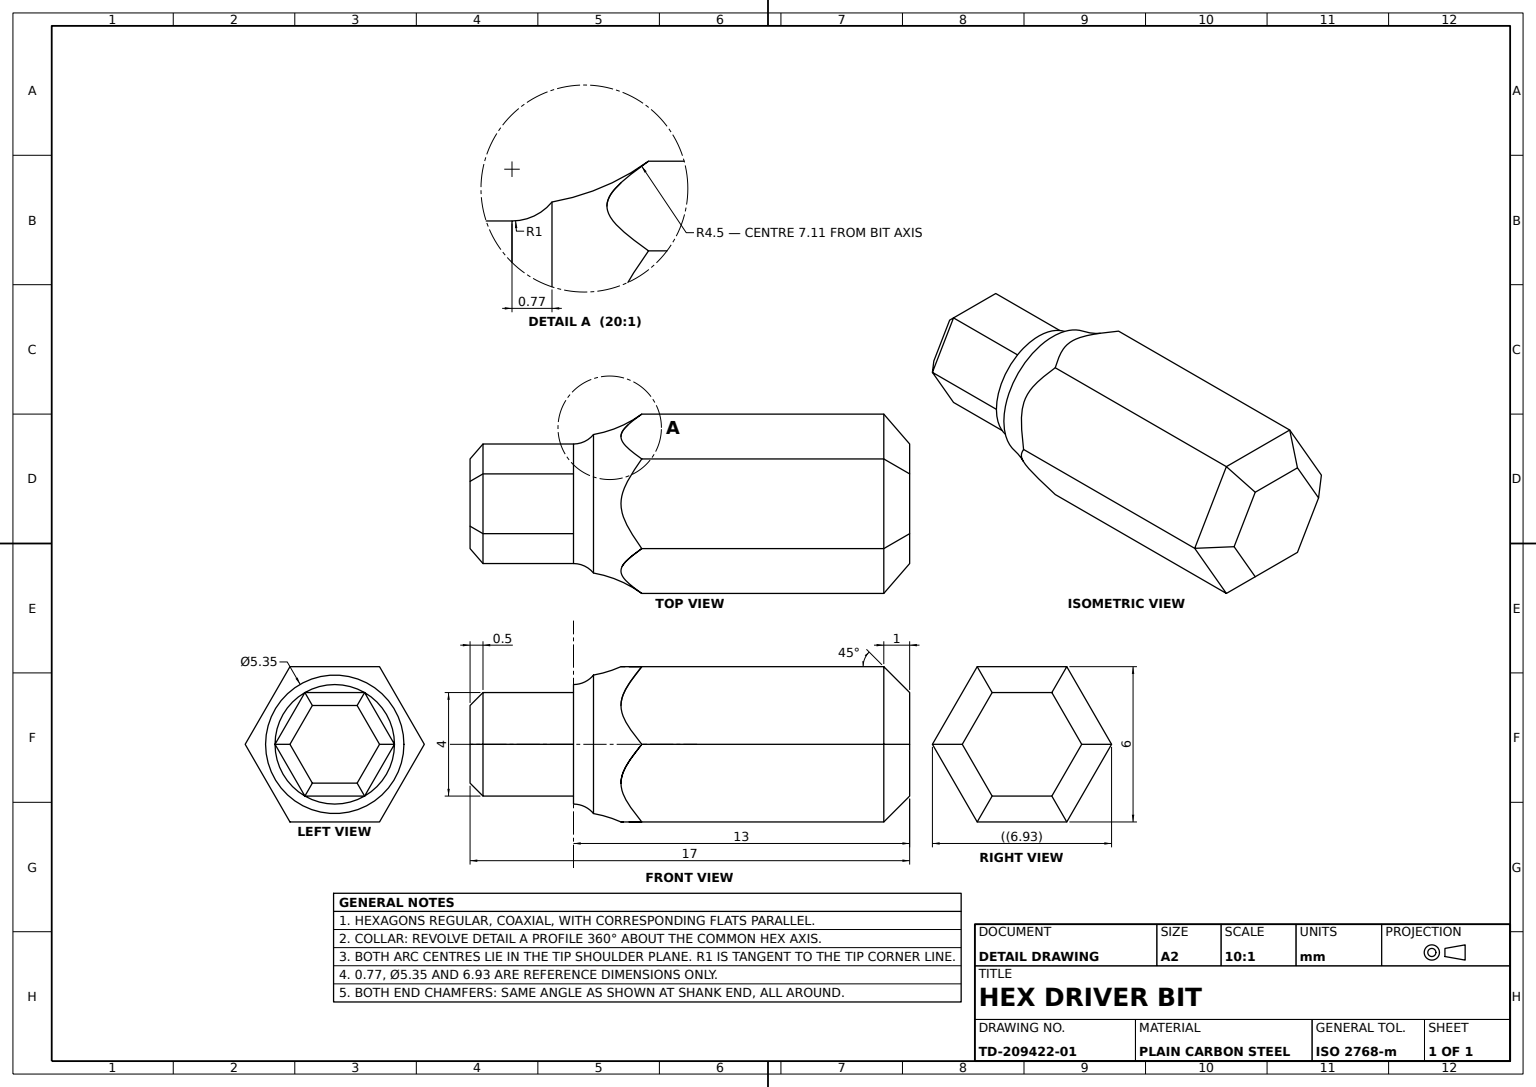
SolidWorks part; units mm, degrees
material "Plain Carbon Steel"
ref_plane "Front Plane" through (0, 0, 0) normal (0, 0, 1) x (1, 0, 0)
ref_plane "Top Plane" through (0, 0, 0) normal (0, 1, 0) x (1, 0, 0)
ref_plane "Right Plane" through (0, 0, 0) normal (1, 0, 0) x (0, 0, -1)
sketch "Hex Shank Profile 6AF" plane through (0, 0, 0) normal (0, 0, 1) x (1, 0, 0)
  line L1 (3.4641, 0) -> (1.7321, 3)
  line L2 (1.7321, 3) -> (-1.7321, 3)
  line L3 (-1.7321, 3) -> (-3.4641, 0)
  line L4 (-3.4641, 0) -> (-1.7321, -3)
  line L5 (-1.7321, -3) -> (1.7321, -3)
  line L6 (1.7321, -3) -> (3.4641, 0)
  circle A0 centre (0, 0) radius 3 construction
  dimension "D1" = 6
extrude "Hex Shank 6AF x13" add sketch "Hex Shank Profile 6AF" along normal blind 13
sketch "Hex Tip Profile 4AF" plane through (0, 0, 13) normal (0, 0, 1) x (1, 0, 0)
  line L1 (2.3094, 0) -> (1.1547, 2)
  line L2 (1.1547, 2) -> (-1.1547, 2)
  line L3 (-1.1547, 2) -> (-2.3094, 0)
  line L4 (-2.3094, 0) -> (-1.1547, -2)
  line L5 (-1.1547, -2) -> (1.1547, -2)
  line L6 (1.1547, -2) -> (2.3094, 0)
  circle A0 centre (0, 0) radius 2 construction
  dimension "D1" = 4
extrude "Hex Tip 4AF x4" add sketch "Hex Tip Profile 4AF" along normal blind 4 and the other way blind 4
sketch "Neck Groove Profile" plane through (0, 0, 0) normal (0, 1, 0) x (1, 0, 0)
  line L4 (3.4641, -10.3601) -> (3.4641, -13)
  line L15 (3.4641, -13) -> (3.4641, 0) construction
  line L32 (0, 0) -> (0, -2.2545) construction
  line L34 (1.1547, -17) -> (2.3094, -17) construction
  line L35 (2.3094, -13) -> (3.4641, -13)
  line L40 (2.3094, -13) -> (2.3094, -17) construction
  arc A1 (2.6753, -12.2267) -> (3.4641, -10.3601) centre (7.1084, -13) cw
  arc A3 (2.6753, -12.2267) -> (2.3094, -13) centre (3.3094, -13) ccw
  dimension "D1" = 4.5
  dimension "D2" = 4
  dimension "D3" = 2
  dimension "D4" = 4
  dimension "D5" = 2.6753
revolve "Neck Groove" cut sketch "Neck Groove Profile" angle 360 about L32
chamfer "Tip Chamfer 0.5" distance 0.5 angle 45 6 edges at (0, -2, 17) (-1.7321, -1, 17) (-1.7321, 1, 17) (0, 2, 17) (1.7321, 1, 17) (1.7321, -1, 17)
chamfer "Shank Chamfer 1" distance 1 angle 45 6 edges at (2.5981, 1.5, 0) (0, 3, 0) (-2.5981, 1.5, 0) (-2.5981, -1.5, 0) (0, -3, 0) (2.5981, -1.5, 0)
